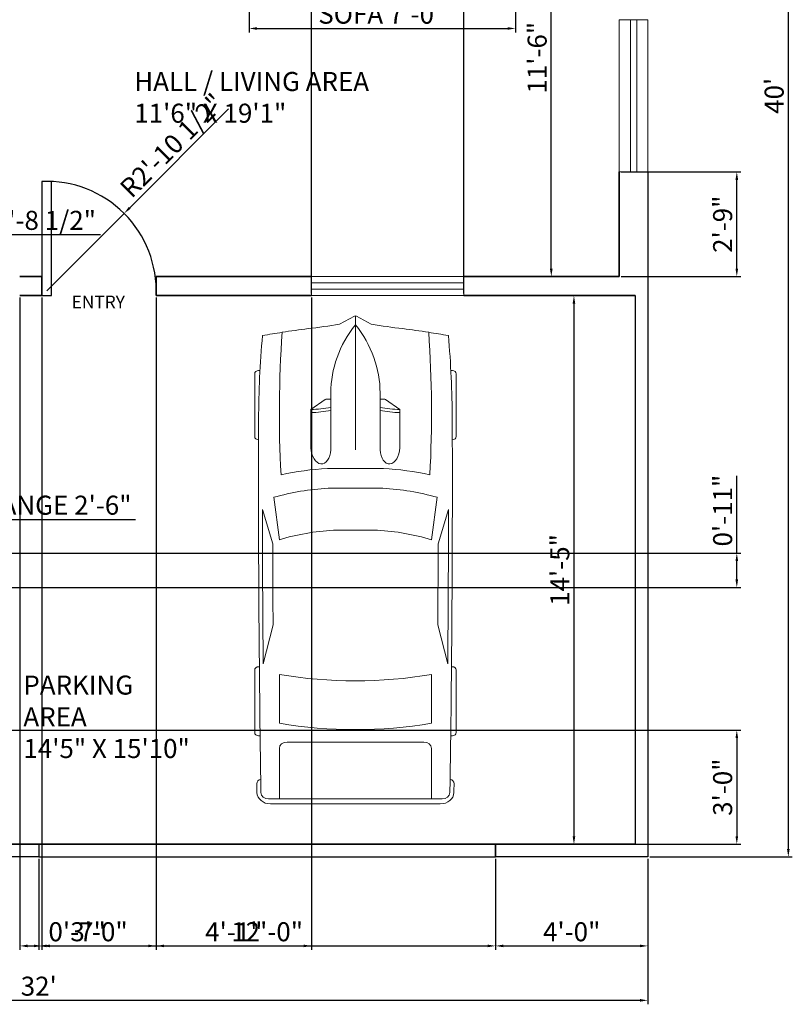
# Model space of a CAD drawing. Units: inches. Extents: x 2117 to 2588, y 1610 to 2201.
# Tile 2 of 4: x 2344 to 2588, y 1610 to 1920. Entities that reach past the tile are written whole.
import ezdxf

# ---------------------------------------------------------------- set-up
doc = ezdxf.new("R2010")
doc.units = ezdxf.units.IN
for name, color, linetype, lineweight in [('A-ANNO-DIMS', 2, 'Continuous', 18), ('A-AREA-IDEN', 7, 'Continuous', 25), ('A-DOOR', 4, 'Continuous', 25), ('A-WALL', 7, 'Continuous', 35), ('C-PRKG-VEHI', 8, 'Continuous', 13), ('C-PROP', 7, 'Continuous', 30), ('GATE', 10, 'Continuous', 25), ('WINDOW', 150, 'Continuous', 18)]:
    doc.layers.add(name, color=color, linetype=linetype, lineweight=lineweight)
doc.styles.get("Standard").update_dxf_attribs({"font": 'arial.ttf'})
doc.dimstyles.new('ISO-25', dxfattribs={"dimtxt": 6, "dimasz": 2.5, "dimexe": 1.25, "dimexo": 0.625, "dimtad": 1, "dimlunit": 3, "dimtxsty": 'Standard', "dimcen": 2.5, "dimadec": 0, "dimazin": 0, "dimtfac": 1, "dimtmove": 0, "dimatfit": 3, "dimfxl": 1, "dimarcsym": 0})

# ---------------------------------------------------------------- blocks, each defined once
blk = doc.blocks.new('*D16')
at = {"layer": 'A-ANNO-DIMS', "color": 0, "lineweight": -2, "transparency": 16777216}
for p, q in [((2532.45, 1977.03), (2510.4, 1977.03)), ((2511.65, 1841.53), (2511.65, 1974.53)), ((2532.45, 1839.03), (2510.4, 1839.03))]:
    blk.add_line(p, q, dxfattribs=at)
at = {"layer": 'A-ANNO-DIMS', "color": 0, "transparency": 16777216}
for points in [[(2511.23, 1974.53), (2512.06, 1974.53), (2511.65, 1977.03)], [(2511.23, 1841.53), (2512.06, 1841.53), (2511.65, 1839.03)]]:
    blk.add_solid(points, dxfattribs=at)
at = {"layer": 'Defpoints', "color": 0, "transparency": 16777216}
for p in [(2511.65, 1977.03), (2533.08, 1977.03), (2533.08, 1839.03)]:
    blk.add_point(p, dxfattribs=at)
at = {"layer": 'A-ANNO-DIMS', "color": 0, "transparency": 16777216, "insert": (2507.96, 1908.03), "char_height": 6, "attachment_point": 5, "rotation": 90}
blk.add_mtext('11\'-6"', dxfattribs=at)
blk = doc.blocks.new('*D17')
at = {"layer": 'A-ANNO-DIMS', "color": 0, "lineweight": -2, "transparency": 16777216}
for p, q in [((2537.45, 1833.03), (2517.54, 1833.03)), ((2518.79, 1830.53), (2518.79, 1662.53)), ((2537.45, 1660.03), (2517.54, 1660.03))]:
    blk.add_line(p, q, dxfattribs=at)
at = {"layer": 'A-ANNO-DIMS', "color": 0, "transparency": 16777216}
for points in [[(2518.38, 1830.53), (2519.21, 1830.53), (2518.79, 1833.03)], [(2518.38, 1662.53), (2519.21, 1662.53), (2518.79, 1660.03)]]:
    blk.add_solid(points, dxfattribs=at)
at = {"layer": 'Defpoints', "color": 0, "transparency": 16777216}
for p in [(2538.08, 1833.03), (2518.79, 1660.03), (2538.08, 1660.03)]:
    blk.add_point(p, dxfattribs=at)
at = {"layer": 'A-ANNO-DIMS', "color": 0, "transparency": 16777216, "insert": (2515.11, 1746.53), "char_height": 6, "attachment_point": 5, "rotation": 90}
blk.add_mtext('14\'-5"', dxfattribs=at)
blk = doc.blocks.new('*U28')
for p, q in [((1182.5, 987.8), (567.7, 987.8)), ((3472.1, 987.8), (4086.9, 987.8)), ((536, 950.2), (536, 935.5)), ((1214.1, 949.7), (1214.1, 950.2)), ((2234.8, 809.5), (1898.9, 912.4)), ((3411.6, 904.3), (3029.9, 807.2)), ((3440.5, 941.7), (3440.5, 950.2)), ((4118.5, 950.2), (4118.5, 934.1)), ((1778.8, 801), (2194.7, 745.5)), ((4736.4, -850.9), (4736.4, 850.9)), ((4785.3, -832.1), (4785.3, 832.1)), ((3515.9, 745.5), (3994.1, 745.5)), ((4736.4, 745.5), (4242, 745.5)), ((4178.7, 670.3), (4178.7, -670.3)), ((819.6, 295.3), (917.7, 436.1)), ((917.7, 436.1), (1293.8, 436.1)), ((756.2, 241.4), (1312.8, 241.4)), ((815.9, 241.4), (815.9, 283.3)), ((1496.5, -273.7), (1496.5, 273.7)), ((1690.4, -267.4), (1690.4, 267.4)), ((2101.5, 215.8), (2101.5, -215.8)), ((4736.4, -267.4), (4736.4, 267.4)), ((83, 155.7), (2.6, 10.3)), ((0, 0), (1312.8, 0)), ((2.6, -10.3), (83, -155.7)), ((756.2, -241.4), (1312.8, -241.4)), ((815.9, -241.4), (815.9, -283.3)), ((819.6, -295.3), (917.7, -436.1)), ((917.7, -436.1), (1293.8, -436.1)), ((2194.7, -745.5), (1778.8, -801)), ((3994.1, -745.5), (3515.9, -745.5)), ((4242, -745.5), (4736.4, -745.5)), ((2234.8, -809.5), (1898.9, -912.4)), ((3411.6, -904.3), (3029.9, -807.2)), ((536, -950.2), (536, -935.5)), ((1214.1, -949.7), (1214.1, -950.2)), ((3440.5, -941.7), (3440.5, -950.2)), ((4118.5, -950.2), (4118.5, -934.1)), ((1182.5, -987.8), (567.7, -987.8)), ((3472.1, -987.8), (4086.9, -987.8))]:
    blk.add_line(p, q)
for centre, major_axis, ratio, start_param, end_param in [((567.7, 950.2), (0, -37.6), 0.842304, 3.141593, 4.712389), ((1182.5, 950.2), (0, 37.6), 0.842304, -1.570796, 0), ((3472.1, 950.2), (0, -37.6), 0.842304, 3.141593, 4.712389), ((4086.9, 950.2), (0, 37.6), 0.842304, -1.570796, 0), ((4588, 910.3), (0, 56.4), 0.842304, -0.013017, 1.249894), ((1637.8, -268131.5), (0, 269121), 0.842304, -0.013397, -0.013017), ((6757.2, -699.1), (0, 7958), 0.842304, 1.367076, 1.39176), ((1046.3, -12467.9), (0, 13417.1), 0.842304, 0.00281, 0.075598), ((1637.8, -268112.7), (0, 269062.9), 0.842304, -0.013397, 0.002797), ((1637.8, -268112.7), (0, -269025.3), 0.842304, 3.133765, 3.140441), ((4673.1, 850.9), (0, -75.2), 0.842304, 1.570796, 3.128196), ((4673.1, 832.1), (0, -133.3), 0.842304, 1.570796, 3.128196), ((3436.4, 136.8), (0, 2077), 0.842304, 1.245306, 1.50788), ((2433, -93125.4), (0, -93935.2), 0.842304, 3.134049, 3.144098), ((6583, -699.1), (0, -7754.7), 0.842304, 4.528606, 4.561838), ((951.8, -15086.6), (0, -15832.5), 0.842304, 3.096046, 3.200911), ((3413.8, 136.8), (0, -2280.3), 0.842304, 4.449482, 4.652344), ((3799.7, 71.1), (0, -2021.3), 0.842304, 4.372215, 4.640744), ((433.9, 0), (0, 3734.3), 0.842304, 4.511394, 4.913384), ((912, 0), (0, 3734.3), 0.842304, 4.511394, 4.913384), ((4242, 670.3), (0, 75.2), 0.842304, 0, 1.570796), ((-5194.2, 1330.9), (0, -6374.4), 0.842304, 1.385369, 1.434372), ((331.1, 432), (0, 696.4), 0.842304, 4.435146, 4.718221), ((360.7, 432), (0, 696.4), 0.842304, 4.435146, 4.718221), ((1290.1, 338.8), (161, -9.1), 0.603834, -1.395552, 1.581315), ((831.8, 283.3), (0, 18.8), 0.842304, 0.879714, 1.570796), ((756.2, -1185.2), (0, 1426.7), 0.842304, 0, 0.590319), ((15.8, 0), (0, -18.8), 0.842304, 4.131459, 5.293319), ((756.2, 1185.2), (0, 1426.7), 0.842304, 2.551274, 3.141593), ((-5194.2, -1330.9), (0, 6374.4), 0.842304, -1.434372, -1.385369), ((831.8, -283.3), (0, -18.8), 0.842304, 4.712389, 5.403472), ((331.1, -432), (0, -696.4), 0.842304, 1.564964, 1.848039), ((360.7, -432), (0, -696.4), 0.842304, 1.564964, 1.848039), ((3413.8, -136.8), (0, -2280.3), 0.842304, -1.510751, -1.307889), ((3436.4, -136.8), (0, -2077), 0.842304, -1.50788, -1.245306), ((3799.7, -71.1), (0, -2021.3), 0.842304, -1.499151, -1.230623), ((6583, 699.1), (0, 7754.7), 0.842304, 1.721348, 1.754579), ((4242, -670.3), (0, -75.2), 0.842304, 4.712389, 6.283185), ((6757.2, 699.1), (0, 7958), 0.842304, 1.749832, 1.774517), ((951.8, 15086.6), (0, -15832.5), 0.842304, -0.059319, 0.045547), ((2433, 93125.4), (0, -93935.2), 0.842304, -0.002505, 0.007544), ((4673.1, -850.9), (0, 75.2), 0.842304, 3.15499, 4.712389), ((4673.1, -832.1), (0, -133.3), 0.842304, 0.013397, 1.570796), ((1046.3, 12467.9), (0, -13417.1), 0.842304, -0.075598, -0.00281), ((567.7, -950.2), (0, 37.6), 0.842304, 1.570796, 3.141593), ((1637.8, 268112.7), (0, 269062.9), 0.842304, 3.138796, 3.15499), ((1182.5, -950.2), (0, -37.6), 0.842304, 0, 1.570796), ((1637.8, 268112.7), (0, -269025.3), 0.842304, 0.001152, 0.007828), ((3472.1, -950.2), (0, -37.6), 0.842304, -1.570796, 0), ((4086.9, -950.2), (0, 37.6), 0.842304, 3.141593, 4.712389), ((4588, -910.3), (0, -56.4), 0.842304, -1.249894, 0.013017), ((1637.8, 268131.5), (0, 269121), 0.842304, 3.15461, 3.15499)]:
    blk.add_ellipse(centre, major_axis=major_axis, ratio=ratio, start_param=start_param, end_param=end_param)
at = {"extrusion": (0, 0, -1)}
blk.add_ellipse((1290.1, -338.8), major_axis=(161, 9.1), ratio=0.603834, start_param=-1.395552, end_param=1.581315, dxfattribs=at)
blk = doc.blocks.new('*D31')
at = {"layer": 'A-ANNO-DIMS', "color": 0, "lineweight": -2, "transparency": 16777216}
for p, q in [((2542.7, 2136.03), (2587.62, 2136.03)), ((2586.37, 2133.53), (2586.37, 1658.53)), ((2542.7, 1656.03), (2587.62, 1656.03))]:
    blk.add_line(p, q, dxfattribs=at)
at = {"layer": 'A-ANNO-DIMS', "color": 0, "transparency": 16777216}
for points in [[(2585.96, 2133.53), (2586.79, 2133.53), (2586.37, 2136.03)], [(2585.96, 1658.53), (2586.79, 1658.53), (2586.37, 1656.03)]]:
    blk.add_solid(points, dxfattribs=at)
at = {"layer": 'Defpoints', "color": 0, "transparency": 16777216}
for p in [(2542.08, 2136.03), (2542.08, 1656.03), (2586.37, 1656.03)]:
    blk.add_point(p, dxfattribs=at)
at = {"layer": 'A-ANNO-DIMS', "color": 0, "transparency": 16777216, "insert": (2582.68, 1896.03), "char_height": 6, "attachment_point": 5, "rotation": 90}
blk.add_mtext("40'", dxfattribs=at)
blk = doc.blocks.new('*D32')
at = {"layer": 'A-ANNO-DIMS', "color": 0, "lineweight": -2, "transparency": 16777216}
for p, q in [((2158.08, 1655.4), (2158.08, 1609.57)), ((2542.08, 1655.4), (2542.08, 1609.57)), ((2539.58, 1610.82), (2160.58, 1610.82))]:
    blk.add_line(p, q, dxfattribs=at)
at = {"layer": 'A-ANNO-DIMS', "color": 0, "transparency": 16777216}
for points in [[(2160.58, 1611.24), (2160.58, 1610.4), (2158.08, 1610.82)], [(2539.58, 1611.24), (2539.58, 1610.4), (2542.08, 1610.82)]]:
    blk.add_solid(points, dxfattribs=at)
at = {"layer": 'Defpoints', "color": 0, "transparency": 16777216}
for p in [(2158.08, 1656.03), (2542.08, 1656.03), (2158.08, 1610.82)]:
    blk.add_point(p, dxfattribs=at)
at = {"layer": 'A-ANNO-DIMS', "color": 0, "transparency": 16777216, "insert": (2350.08, 1614.51), "char_height": 6, "attachment_point": 5}
blk.add_mtext("32'", dxfattribs=at)
blk = doc.blocks.new('WIN-48IN-9IN-WALL')
for p, q in [((9, 48), (0, 48)), ((0, 0), (0, 48)), ((3.5, 0), (3.5, 48)), ((5.5, 0), (5.5, 48)), ((9, 0), (9, 48)), ((9, 0), (0, 0))]:
    blk.add_line(p, q)
blk = doc.blocks.new('*D49')
at = {"layer": 'A-ANNO-DIMS', "color": 0, "lineweight": -2, "transparency": 16777216}
for p, q in [((2416.37, 1929.23), (2416.37, 1916.01)), ((2500.37, 1929.23), (2500.37, 1916.01)), ((2418.87, 1917.26), (2497.87, 1917.26))]:
    blk.add_line(p, q, dxfattribs=at)
at = {"layer": 'A-ANNO-DIMS', "color": 0, "transparency": 16777216}
for points in [[(2418.87, 1917.67), (2418.87, 1916.84), (2416.37, 1917.26)], [(2497.87, 1917.67), (2497.87, 1916.84), (2500.37, 1917.26)]]:
    blk.add_solid(points, dxfattribs=at)
at = {"layer": 'Defpoints', "color": 0, "transparency": 16777216}
for p in [(2416.37, 1929.86), (2500.37, 1929.86), (2500.37, 1917.26)]:
    blk.add_point(p, dxfattribs=at)
at = {"layer": 'A-ANNO-DIMS', "color": 0, "transparency": 16777216, "insert": (2458.37, 1920.99), "char_height": 6, "attachment_point": 5}
blk.add_mtext('SOFA 7\'-0"', dxfattribs=at)
blk = doc.blocks.new('*D51')
at = {"layer": 'A-ANNO-DIMS', "color": 0, "lineweight": -2, "transparency": 16777216}
for p, q in [((2229.55, 1860.07), (2229.55, 1851)), ((2285.85, 1860.07), (2285.85, 1851)), ((2232.05, 1852.25), (2283.35, 1852.25)), ((2285.85, 1852.25), (2369.53, 1852.25))]:
    blk.add_line(p, q, dxfattribs=at)
at = {"layer": 'A-ANNO-DIMS', "color": 0, "transparency": 16777216}
for points in [[(2232.05, 1852.67), (2232.05, 1851.83), (2229.55, 1852.25)], [(2283.35, 1852.67), (2283.35, 1851.83), (2285.85, 1852.25)]]:
    blk.add_solid(points, dxfattribs=at)
at = {"layer": 'Defpoints', "color": 0, "transparency": 16777216}
for p in [(2229.55, 1860.69), (2285.85, 1860.69), (2285.85, 1852.25)]:
    blk.add_point(p, dxfattribs=at)
at = {"layer": 'A-ANNO-DIMS', "color": 0, "transparency": 16777216, "insert": (2328.94, 1855.98), "char_height": 6, "attachment_point": 5}
blk.add_mtext('DINING SET 4\'-8 1/2"', dxfattribs=at)
blk = doc.blocks.new('*D53')
at = {"layer": 'A-ANNO-DIMS', "color": 0, "lineweight": -2, "transparency": 16777216}
for p, q in [((2299.08, 1766.32), (2299.08, 1761.19)), ((2329.08, 1766.32), (2329.08, 1761.19)), ((2301.58, 1762.44), (2326.58, 1762.44)), ((2329.08, 1762.44), (2380.6, 1762.44))]:
    blk.add_line(p, q, dxfattribs=at)
at = {"layer": 'A-ANNO-DIMS', "color": 0, "transparency": 16777216}
for points in [[(2301.58, 1762.86), (2301.58, 1762.02), (2299.08, 1762.44)], [(2326.58, 1762.86), (2326.58, 1762.02), (2329.08, 1762.44)]]:
    blk.add_solid(points, dxfattribs=at)
at = {"layer": 'Defpoints', "color": 0, "transparency": 16777216}
for p in [(2299.08, 1766.94), (2329.08, 1766.94), (2329.08, 1762.44)]:
    blk.add_point(p, dxfattribs=at)
at = {"layer": 'A-ANNO-DIMS', "color": 0, "transparency": 16777216, "insert": (2356.09, 1766.17), "char_height": 6, "attachment_point": 5}
blk.add_mtext('RANGE 2\'-6"', dxfattribs=at)
blk = doc.blocks.new('*D57')
at = {"layer": 'A-ANNO-DIMS', "color": 0, "lineweight": -2, "transparency": 16777216}
for p, q in [((2351.08, 1832.4), (2351.08, 1626.73)), ((2387.08, 1832.4), (2387.08, 1626.73)), ((2353.58, 1627.98), (2384.58, 1627.98))]:
    blk.add_line(p, q, dxfattribs=at)
at = {"layer": 'A-ANNO-DIMS', "color": 0, "transparency": 16777216}
for points in [[(2353.58, 1628.4), (2353.58, 1627.56), (2351.08, 1627.98)], [(2384.58, 1628.4), (2384.58, 1627.56), (2387.08, 1627.98)]]:
    blk.add_solid(points, dxfattribs=at)
at = {"layer": 'Defpoints', "color": 0, "transparency": 16777216}
for p in [(2351.08, 1833.03), (2387.08, 1833.03), (2387.08, 1627.98)]:
    blk.add_point(p, dxfattribs=at)
at = {"layer": 'A-ANNO-DIMS', "color": 0, "transparency": 16777216, "insert": (2369.08, 1631.67), "char_height": 6, "attachment_point": 5}
blk.add_mtext('3\'-0"', dxfattribs=at)
blk = doc.blocks.new('*D59')
at = {"layer": 'A-ANNO-DIMS', "color": 0, "lineweight": -2, "transparency": 16777216}
for p, q in [((2319.7, 1696.03), (2571.38, 1696.03)), ((2570.13, 1693.53), (2570.13, 1662.53)), ((2319.7, 1660.03), (2571.38, 1660.03))]:
    blk.add_line(p, q, dxfattribs=at)
at = {"layer": 'A-ANNO-DIMS', "color": 0, "transparency": 16777216}
for points in [[(2569.71, 1693.53), (2570.54, 1693.53), (2570.13, 1696.03)], [(2569.71, 1662.53), (2570.54, 1662.53), (2570.13, 1660.03)]]:
    blk.add_solid(points, dxfattribs=at)
at = {"layer": 'Defpoints', "color": 0, "transparency": 16777216}
for p in [(2319.08, 1696.03), (2319.08, 1660.03), (2570.13, 1660.03)]:
    blk.add_point(p, dxfattribs=at)
at = {"layer": 'A-ANNO-DIMS', "color": 0, "transparency": 16777216, "insert": (2566.44, 1678.03), "char_height": 6, "attachment_point": 5, "rotation": 90}
blk.add_mtext('3\'-0"', dxfattribs=at)
blk = doc.blocks.new('*D66')
at = {"layer": 'A-ANNO-DIMS', "color": 0, "lineweight": -2, "transparency": 16777216}
for p, q in [((2533.7, 1872.03), (2571.38, 1872.03)), ((2570.13, 1841.53), (2570.13, 1869.53)), ((2533.7, 1839.03), (2571.38, 1839.03))]:
    blk.add_line(p, q, dxfattribs=at)
at = {"layer": 'A-ANNO-DIMS', "color": 0, "transparency": 16777216}
for points in [[(2569.71, 1869.53), (2570.54, 1869.53), (2570.13, 1872.03)], [(2569.71, 1841.53), (2570.54, 1841.53), (2570.13, 1839.03)]]:
    blk.add_solid(points, dxfattribs=at)
at = {"layer": 'Defpoints', "color": 0, "transparency": 16777216}
for p in [(2533.08, 1872.03), (2570.13, 1872.03), (2533.08, 1839.03)]:
    blk.add_point(p, dxfattribs=at)
at = {"layer": 'A-ANNO-DIMS', "color": 0, "transparency": 16777216, "insert": (2566.44, 1855.53), "char_height": 6, "attachment_point": 5, "rotation": 90}
blk.add_mtext('2\'-9"', dxfattribs=at)
blk = doc.blocks.new('*D67')
at = {"layer": 'A-ANNO-DIMS', "color": 0, "lineweight": -2, "transparency": 16777216}
for p, q in [((2387.08, 1832.4), (2387.08, 1626.73)), ((2436.08, 1832.4), (2436.08, 1626.73)), ((2389.58, 1627.98), (2433.58, 1627.98))]:
    blk.add_line(p, q, dxfattribs=at)
at = {"layer": 'A-ANNO-DIMS', "color": 0, "transparency": 16777216}
for points in [[(2389.58, 1628.4), (2389.58, 1627.56), (2387.08, 1627.98)], [(2433.58, 1628.4), (2433.58, 1627.56), (2436.08, 1627.98)]]:
    blk.add_solid(points, dxfattribs=at)
at = {"layer": 'Defpoints', "color": 0, "transparency": 16777216}
for p in [(2387.08, 1833.03), (2436.08, 1833.03), (2436.08, 1627.98)]:
    blk.add_point(p, dxfattribs=at)
at = {"layer": 'A-ANNO-DIMS', "color": 0, "transparency": 16777216, "insert": (2411.58, 1631.62), "char_height": 6, "attachment_point": 5}
blk.add_mtext('4\'-1"', dxfattribs=at)
blk = doc.blocks.new('*D69')
at = {"layer": 'A-ANNO-DIMS', "color": 0, "lineweight": -2, "transparency": 16777216}
for p, q in [((2570.13, 1751.81), (2570.13, 1776.17)), ((2335.7, 1751.81), (2571.38, 1751.81)), ((2570.13, 1743.53), (2570.13, 1749.31)), ((2335.7, 1741.03), (2571.38, 1741.03))]:
    blk.add_line(p, q, dxfattribs=at)
at = {"layer": 'A-ANNO-DIMS', "color": 0, "transparency": 16777216}
for points in [[(2569.71, 1749.31), (2570.54, 1749.31), (2570.13, 1751.81)], [(2569.71, 1743.53), (2570.54, 1743.53), (2570.13, 1741.03)]]:
    blk.add_solid(points, dxfattribs=at)
at = {"layer": 'Defpoints', "color": 0, "transparency": 16777216}
for p in [(2335.08, 1751.81), (2570.13, 1751.81), (2335.08, 1741.03)]:
    blk.add_point(p, dxfattribs=at)
at = {"layer": 'A-ANNO-DIMS', "color": 0, "transparency": 16777216, "insert": (2566.44, 1765.24), "char_height": 6, "attachment_point": 5, "rotation": 90}
blk.add_mtext('0\'-11"', dxfattribs=at)
blk = doc.blocks.new('*D72')
at = {"layer": 'A-ANNO-DIMS', "color": 0, "lineweight": -2, "transparency": 16777216}
for p, q in [((2350.08, 1655.4), (2350.08, 1626.73)), ((2494.08, 1655.4), (2494.08, 1626.73)), ((2352.58, 1627.98), (2491.58, 1627.98))]:
    blk.add_line(p, q, dxfattribs=at)
at = {"layer": 'A-ANNO-DIMS', "color": 0, "transparency": 16777216}
for points in [[(2352.58, 1628.4), (2352.58, 1627.56), (2350.08, 1627.98)], [(2491.58, 1628.4), (2491.58, 1627.56), (2494.08, 1627.98)]]:
    blk.add_solid(points, dxfattribs=at)
at = {"layer": 'Defpoints', "color": 0, "transparency": 16777216}
for p in [(2350.08, 1656.03), (2494.08, 1656.03), (2494.08, 1627.98)]:
    blk.add_point(p, dxfattribs=at)
at = {"layer": 'A-ANNO-DIMS', "color": 0, "transparency": 16777216, "insert": (2422.08, 1631.67), "char_height": 6, "attachment_point": 5}
blk.add_mtext('12\'-0"', dxfattribs=at)
blk = doc.blocks.new('*D73')
at = {"layer": 'A-ANNO-DIMS', "color": 0, "lineweight": -2, "transparency": 16777216}
for p, q in [((2494.08, 1655.4), (2494.08, 1626.73)), ((2542.08, 1655.4), (2542.08, 1626.73)), ((2496.58, 1627.98), (2539.58, 1627.98))]:
    blk.add_line(p, q, dxfattribs=at)
at = {"layer": 'A-ANNO-DIMS', "color": 0, "transparency": 16777216}
for points in [[(2496.58, 1628.4), (2496.58, 1627.56), (2494.08, 1627.98)], [(2539.58, 1628.4), (2539.58, 1627.56), (2542.08, 1627.98)]]:
    blk.add_solid(points, dxfattribs=at)
at = {"layer": 'Defpoints', "color": 0, "transparency": 16777216}
for p in [(2494.08, 1656.03), (2542.08, 1656.03), (2542.08, 1627.98)]:
    blk.add_point(p, dxfattribs=at)
at = {"layer": 'A-ANNO-DIMS', "color": 0, "transparency": 16777216, "insert": (2518.08, 1631.67), "char_height": 6, "attachment_point": 5}
blk.add_mtext('4\'-0"', dxfattribs=at)
blk = doc.blocks.new('*D74')
at = {"layer": 'A-ANNO-DIMS', "color": 0, "lineweight": -2, "transparency": 16777216}
for p, q in [((2344.08, 1832.4), (2344.08, 1626.73)), ((2351.08, 1832.4), (2351.08, 1626.73)), ((2346.58, 1627.98), (2348.58, 1627.98)), ((2351.08, 1627.98), (2370.78, 1627.98))]:
    blk.add_line(p, q, dxfattribs=at)
at = {"layer": 'A-ANNO-DIMS', "color": 0, "transparency": 16777216}
for points in [[(2346.58, 1628.4), (2346.58, 1627.56), (2344.08, 1627.98)], [(2348.58, 1628.4), (2348.58, 1627.56), (2351.08, 1627.98)]]:
    blk.add_solid(points, dxfattribs=at)
at = {"layer": 'Defpoints', "color": 0, "transparency": 16777216}
for p in [(2344.08, 1833.03), (2351.08, 1833.03), (2351.08, 1627.98)]:
    blk.add_point(p, dxfattribs=at)
at = {"layer": 'A-ANNO-DIMS', "color": 0, "transparency": 16777216, "insert": (2362.18, 1631.67), "char_height": 6, "attachment_point": 5}
blk.add_mtext('0\'-7"', dxfattribs=at)
blk = doc.blocks.new('*D75')
at = {"layer": 'A-ANNO-DIMS', "color": 0, "lineweight": -2, "transparency": 16777216}
for p, q in [((2436.08, 1833.65), (2436.08, 2165.33)), ((2438.58, 2164.08), (2481.58, 2164.08)), ((2484.08, 1833.65), (2484.08, 2165.33))]:
    blk.add_line(p, q, dxfattribs=at)
at = {"layer": 'A-ANNO-DIMS', "color": 0, "transparency": 16777216}
for points in [[(2438.58, 2164.5), (2438.58, 2163.66), (2436.08, 2164.08)], [(2481.58, 2164.5), (2481.58, 2163.66), (2484.08, 2164.08)]]:
    blk.add_solid(points, dxfattribs=at)
at = {"layer": 'Defpoints', "color": 0, "transparency": 16777216}
for p in [(2484.08, 2164.08), (2436.08, 1833.03), (2484.08, 1833.03)]:
    blk.add_point(p, dxfattribs=at)
at = {"layer": 'A-ANNO-DIMS', "color": 0, "transparency": 16777216, "insert": (2460.08, 2167.77), "char_height": 6, "attachment_point": 5}
blk.add_mtext('4\'-0"', dxfattribs=at)
blk = doc.blocks.new('*D77')
at = {"layer": 'A-ANNO-DIMS', "color": 0, "lineweight": -2, "transparency": 16777216}
for p, q in [((2409.93, 1891.89), (2378.76, 1860.71)), ((2352.58, 1834.53), (2376.99, 1858.95))]:
    blk.add_line(p, q, dxfattribs=at)
at = {"layer": 'A-ANNO-DIMS', "color": 0, "transparency": 16777216}
blk.add_solid([(2378.47, 1861.01), (2379.06, 1860.42), (2376.99, 1858.95)], dxfattribs=at)
at = {"layer": 'Defpoints', "color": 0, "transparency": 16777216}
for p in [(2376.99, 1858.95), (2352.58, 1834.53)]:
    blk.add_point(p, dxfattribs=at)
at = {"layer": 'A-ANNO-DIMS', "color": 0, "transparency": 16777216, "insert": (2392.6, 1879.82), "char_height": 6, "attachment_point": 5, "rotation": 45.0004}
blk.add_mtext('R2\'-10 1/2"', dxfattribs=at)

msp = doc.modelspace()

# ---------------------------------------------------------------- linework, layer by layer
at = {"layer": 'A-DOOR'}
msp.add_lwpolyline([(2351.076, 1833.029), (2354.076, 1833.029), (2354.076, 1869.029), (2351.076, 1869.029)], close=True, dxfattribs=at)
msp.add_arc((2352.576, 1834.529), 34.533, 357.51045, 92.48955, dxfattribs=at)
at = {"layer": 'A-WALL'}
for p, q in [((2533.076, 1872.029), (2533.076, 1839.029)), ((2344.076, 1839.029), (2351.076, 1839.029)), ((2351.076, 1833.029), (2351.076, 1839.029)), ((2387.076, 1833.029), (2387.076, 1839.029)), ((2387.076, 1839.029), (2436.076, 1839.029)), ((2484.076, 1839.029), (2533.076, 1839.029)), ((2344.076, 1833.029), (2351.076, 1833.029)), ((2351.076, 1833.029), (2344.076, 1833.029)), ((2436.076, 1833.029), (2387.076, 1833.029)), ((2538.076, 1833.029), (2484.076, 1833.029))]:
    msp.add_line(p, q, dxfattribs=at)
at = {"layer": 'C-PROP'}
for p, q in [((2538.076, 1833.029), (2538.076, 1660.029)), ((2350.076, 1660.029), (2162.076, 1660.029)), ((2350.076, 1660.029), (2350.076, 1656.029)), ((2538.076, 1660.029), (2494.076, 1660.029)), ((2494.076, 1660.029), (2494.076, 1656.029))]:
    msp.add_line(p, q, dxfattribs=at)
for points in [[(2350.076, 1656.029), (2158.076, 1656.029), (2158.076, 2136.029), (2361.076, 2136.029)], [(2542.076, 1872.029), (2542.076, 1656.029), (2494.076, 1656.029)]]:
    msp.add_lwpolyline(points, dxfattribs=at)
at = {"layer": 'GATE'}
for p, q in [((2494.076, 1660.029), (2350.076, 1660.029)), ((2350.076, 1660.029), (2350.076, 1656.029)), ((2494.076, 1656.029), (2494.076, 1660.029)), ((2350.076, 1656.029), (2494.076, 1656.029))]:
    msp.add_line(p, q, dxfattribs=at)
at = {"layer": 'WINDOW'}
for p, q in [((2436.076, 1839.029), (2436.076, 1833.029)), ((2436.076, 1839.029), (2484.076, 1839.029)), ((2484.076, 1839.029), (2484.076, 1833.029)), ((2436.076, 1837.029), (2484.076, 1837.029)), ((2436.076, 1835.029), (2484.076, 1835.029)), ((2484.076, 1833.029), (2436.076, 1833.029))]:
    msp.add_line(p, q, dxfattribs=at)

# ---------------------------------------------------------------- block references
at = {"layer": 'C-PRKG-VEHI', "xscale": 0.0321563088240144, "yscale": 0.0321563088240144, "zscale": 0.0321563088240144, "rotation": 270}
msp.add_blockref('*U28', (2449.909, 1826.642), dxfattribs=at)
at = {"layer": 'WINDOW', "rotation": 180}
msp.add_blockref('WIN-48IN-9IN-WALL', (2542.076, 1920.028), dxfattribs=at)

# ---------------------------------------------------------------- texts
at = {"layer": 'A-AREA-IDEN', "attachment_point": 1}
for s, width, insert, char_height in [('{\\fArial|b1|i0|c0|p34;HALL / LIVING AREA \\P11\'6" X 19\'1"}', 117.5236, (2380.193, 1903.543), 6), ('{\\fArial|b1|i0|c0|p34;ENTRY }', 34.92104, (2360.455, 1833.029), 4), ('{\\fArial|b1|i0|c0|p34;PARKING AREA \\P14\'5" X 15\'10"}', 54.84913, (2345.238, 1713.222), 6)]:
    msp.add_mtext_dynamic_manual_height_columns(s, width=width, gutter_width=12.5, heights=[0], dxfattribs=dict(at, insert=insert, char_height=char_height))

# ---------------------------------------------------------------- dimensions: what is measured, and where the dimension line sits
at = {"layer": 'A-ANNO-DIMS'}
for base, p1, p2, override, picture, middle in [((2484.076, 2164.079), (2436.076, 1833.029), (2484.076, 1833.029), {"dimdec": 1, "dimlfac": 1, "dimrnd": 0, "dimzin": 1, "dimdsep": 46, "dimlunit": 4, "dimfrac": 2}, '*D75', (2460.076, 2167.767)), ((2351.076, 1627.979), (2344.076, 1833.029), (2351.076, 1833.029), {"dimdec": 1, "dimlfac": 1, "dimrnd": 0, "dimzin": 1, "dimdsep": 46, "dimlunit": 4, "dimfrac": 2}, '*D74', (2362.176, 1631.667)), ((2387.076, 1627.979), (2351.076, 1833.029), (2387.076, 1833.029), {"dimdec": 1, "dimlfac": 1, "dimrnd": 0, "dimzin": 1, "dimdsep": 46, "dimlunit": 4, "dimfrac": 2}, '*D57', (2369.076, 1631.669)), ((2436.076, 1627.979), (2387.076, 1833.029), (2436.076, 1833.029), {"dimdec": 1, "dimlfac": 1, "dimrnd": 0, "dimzin": 1, "dimdsep": 46, "dimlunit": 4, "dimfrac": 2}, '*D67', (2411.576, 1631.616)), ((2158.076, 1610.819), (2542.076, 1656.029), (2158.076, 1656.029), {"dimclrd": 0, "dimclre": 0, "dimclrt": 0}, '*D32', (2350.076, 1614.509)), ((2494.076, 1627.979), (2350.076, 1656.029), (2494.076, 1656.029), {"dimdec": 1, "dimlfac": 1, "dimrnd": 0, "dimzin": 1, "dimdsep": 46, "dimlunit": 4, "dimfrac": 2}, '*D72', (2422.076, 1631.667)), ((2542.076, 1627.979), (2494.076, 1656.029), (2542.076, 1656.029), {"dimdec": 1, "dimlfac": 1, "dimrnd": 0, "dimzin": 1, "dimdsep": 46, "dimlunit": 4, "dimfrac": 2}, '*D73', (2518.076, 1631.667))]:
    dim = msp.add_linear_dim(base=base, p1=p1, p2=p2, dimstyle='ISO-25', override=override, dxfattribs=at)
    dim.commit()
    dim.dimension.update_dxf_attribs({"geometry": picture, "text_midpoint": middle})
for base, p1, p2, override, picture, middle in [((2586.372, 1656.029), (2542.076, 2136.029), (2542.076, 1656.029), {"dimclrd": 0, "dimclre": 0, "dimclrt": 0}, '*D31', (2582.684, 1896.029)), ((2511.647, 1977.029), (2533.076, 1839.029), (2533.076, 1977.029), {"dimclrd": 0, "dimclre": 0, "dimclrt": 0}, '*D16', (2507.958, 1908.029)), ((2570.126, 1872.029), (2533.076, 1839.029), (2533.076, 1872.029), {"dimdec": 1, "dimlfac": 1, "dimrnd": 0, "dimzin": 1, "dimdsep": 46, "dimlunit": 4, "dimfrac": 2}, '*D66', (2566.437, 1855.529)), ((2518.794, 1660.029), (2538.076, 1833.029), (2538.076, 1660.029), {"dimclrd": 0, "dimclre": 0, "dimclrt": 0}, '*D17', (2515.105, 1746.529)), ((2570.126, 1751.807), (2335.076, 1741.029), (2335.076, 1751.807), {"dimdec": 1, "dimlfac": 1, "dimrnd": 0, "dimzin": 1, "dimdsep": 46, "dimlunit": 4, "dimfrac": 2}, '*D69', (2566.437, 1765.237)), ((2570.126, 1660.029), (2319.076, 1696.029), (2319.076, 1660.029), {"dimdec": 1, "dimlfac": 1, "dimrnd": 0, "dimzin": 1, "dimdsep": 46, "dimlunit": 4, "dimfrac": 2}, '*D59', (2566.435, 1678.029))]:
    dim = msp.add_linear_dim(base=base, p1=p1, p2=p2, angle=90, dimstyle='ISO-25', override=override, dxfattribs=at)
    dim.commit()
    dim.dimension.update_dxf_attribs({"geometry": picture, "text_midpoint": middle})
for base, p1, p2, text, picture, middle in [((2500.372, 1917.256), (2416.372, 1929.856), (2500.372, 1929.856), 'SOFA <>', '*D49', (2458.372, 1920.986)), ((2285.848, 1852.249), (2229.554, 1860.694), (2285.848, 1860.694), 'DINING SET <>', '*D51', (2328.937, 1855.977)), ((2329.076, 1762.441), (2299.076, 1766.941), (2329.076, 1766.941), 'RANGE <>', '*D53', (2356.088, 1766.169))]:
    dim = msp.add_linear_dim(base=base, p1=p1, p2=p2, text=text, dimstyle='ISO-25', override={"dimdec": 1, "dimlfac": 1, "dimrnd": 0, "dimzin": 1, "dimdsep": 46, "dimlunit": 4, "dimfrac": 2}, dxfattribs=at)
    dim.commit()
    dim.dimension.update_dxf_attribs({"geometry": picture, "text_midpoint": middle})
dim = msp.add_radius_dim(center=(2352.576, 1834.529), mpoint=(2376.994, 1858.947), dimstyle='ISO-25', override={"dimdec": 1, "dimlfac": 1, "dimrnd": 0, "dimzin": 1, "dimdsep": 46, "dimlunit": 4, "dimfrac": 2}, dxfattribs=at)
dim.commit()
dim.dimension.update_dxf_attribs({"geometry": '*D77', "text_midpoint": (2392.596, 1879.82)})

doc.saveas('drawing.dxf')
